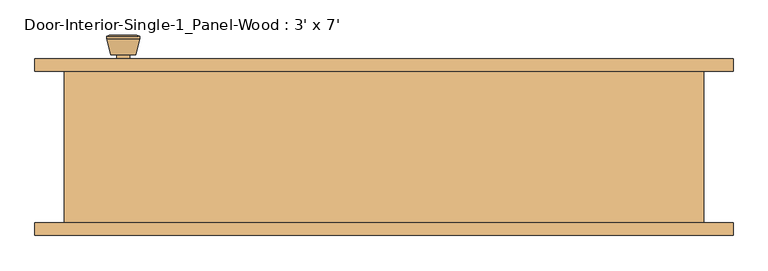
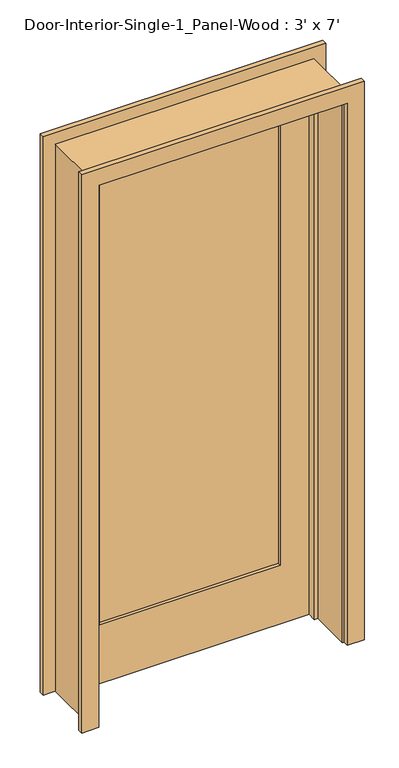
"""IFC4 building model written with IfcOpenShell, lengths in millimetres: door geometry, Door-Interior-Single-1_Panel-Wood : 3' x 7'."""

from ifc_helpers import new_model, si_unit, point, frame, frame_2d, origin, place, context, project, spatial, polyline, circle_curve, trimmed, segment, composite_curve, outline, extrude, faceted_brep, source, transform, mapped, element, save
from ifc_brep_helpers import plane_surface, cylinder_surface, revolved_surface, advanced_brep


def door_interior_single_1_panel_wood_3_x_7_3b97b8e7(model_context):
    return source(origin(), model_context, "Body", "SolidModel", [
        advanced_brep(
        [(-393.7, 70.2, 914.4), (-383.7, 70.2, 914.4), (-403.7, 70.2, 914.4), (-373.2241324, 21.2, 914.4), (-393.7, 21.2, 914.4), (-414.1758676, 21.2, 914.4), (-368.7, 23.0278681, 914.4), (-418.7, 23.0278681, 914.4), (-368.7, 26.4915463, 914.4), (-418.7, 26.4915463, 914.4), (-375.063764, 51.2, 914.4), (-412.336236, 51.2, 914.4), (-383.7, 51.2, 914.4), (-403.7, 51.2, 914.4)],
        [
            (0, 1),
            (1, 2, circle_curve(frame((-393.7, 70.2, 914.4), z_axis=(0.0, 1.0, 0.0), x_axis=(-1.0, 0.0, 0.0)), 10.0)),
            (2, 0),
            (2, 1, circle_curve(frame((-393.7, 70.2, 914.4), z_axis=(0.0, 1.0, 0.0), x_axis=(-1.0, 0.0, 0.0)), 10.0)),
            (3, 4),
            (4, 5),
            (5, 3, circle_curve(frame((-393.7, 21.2, 914.4), z_axis=(0.0, -1.0, 0.0), x_axis=(-1.0, 0.0, 0.0)), 20.4758676)),
            (3, 5, circle_curve(frame((-393.7, 21.2, 914.4), z_axis=(0.0, -1.0, 0.0), x_axis=(-1.0, 0.0, 0.0)), 20.4758676)),
            (6, 3),
            (5, 7),
            (7, 6, circle_curve(frame((-393.7, 23.0278681, 914.4), z_axis=(0.0, -1.0, 0.0), x_axis=(-1.0, 0.0, 0.0)), 25.0)),
            (6, 7, circle_curve(frame((-393.7, 23.0278681, 914.4), z_axis=(0.0, -1.0, 0.0), x_axis=(-1.0, 0.0, 0.0)), 25.0)),
            (8, 6),
            (7, 9),
            (9, 8, circle_curve(frame((-393.7, 26.4915463, 914.4), z_axis=(0.0, -1.0, 0.0), x_axis=(-1.0, 0.0, 0.0)), 25.0)),
            (8, 9, circle_curve(frame((-393.7, 26.4915463, 914.4), z_axis=(0.0, -1.0, 0.0), x_axis=(-1.0, 0.0, 0.0)), 25.0)),
            (10, 8),
            (9, 11),
            (11, 10, circle_curve(frame((-393.7, 51.2, 914.4), z_axis=(0.0, -1.0, 0.0), x_axis=(-1.0, 0.0, 0.0)), 18.636236)),
            (10, 11, circle_curve(frame((-393.7, 51.2, 914.4), z_axis=(0.0, -1.0, 0.0), x_axis=(-1.0, 0.0, 0.0)), 18.636236)),
            (12, 10),
            (11, 13),
            (13, 12, circle_curve(frame((-393.7, 51.2, 914.4), z_axis=(0.0, -1.0, 0.0), x_axis=(-1.0, 0.0, 0.0)), 10.0)),
            (12, 13, circle_curve(frame((-393.7, 51.2, 914.4), z_axis=(0.0, -1.0, 0.0), x_axis=(-1.0, 0.0, 0.0)), 10.0)),
            (1, 12),
            (13, 2),
        ],
        [
            plane_surface(frame((-393.7, 70.2, 914.4), z_axis=(0.0, 1.0, 0.0), x_axis=(-1.0, 0.0, 0.0))),
            plane_surface(frame((-393.7, 21.2, 914.4), z_axis=(0.0, -1.0, 0.0), x_axis=(-1.0, 0.0, 0.0))),
            revolved_surface(polyline([(-414.1758676, 21.2, 914.4), (-418.7, 23.0278681, 914.4)]), (-393.7, 70.2, 914.4), (0.0, 1.0, 0.0)),
            cylinder_surface(frame((-393.7, 70.2, 914.4), z_axis=(0.0, 1.0, 0.0), x_axis=(-1.0, 0.0, 0.0)), 25.0),
            revolved_surface(polyline([(-418.7, 26.4915463, 914.4), (-412.336236, 51.2, 914.4)]), (-393.7, 70.2, 914.4), (0.0, 1.0, 0.0)),
            plane_surface(frame((-393.7, 51.2, 914.4), z_axis=(0.0, 1.0, 0.0), x_axis=(-1.0, 0.0, 0.0))),
            cylinder_surface(frame((-393.7, 70.2, 914.4), z_axis=(0.0, 1.0, 0.0), x_axis=(-1.0, 0.0, 0.0)), 10.0),
        ],
        [
            (0, [[1, 2, 3]]),
            (0, [[-3, 4, -1]]),
            (1, [[5, 6, 7]]),
            (1, [[-6, -5, 8]]),
            (2, [[9, -7, 10, 11]]),
            (2, [[-10, -8, -9, 12]]),
            (3, [[13, -11, 14, 15]]),
            (3, [[-14, -12, -13, 16]]),
            (4, [[17, -15, 18, 19]]),
            (4, [[-18, -16, -17, 20]]),
            (5, [[21, -19, 22, 23]]),
            (5, [[-22, -20, -21, 24]]),
            (6, [[25, -23, 26, -2]]),
            (6, [[-26, -24, -25, -4]]),
        ],
    ),
        extrude(outline(composite_curve([segment(trimmed(circle_curve(frame_2d((914.4, -393.7)), 30.0), [point((914.4, -423.7))], [point((914.4, -363.7))], False, "CARTESIAN"), True, "CONTINUOUS"), segment(trimmed(circle_curve(frame_2d((914.4, -393.7)), 30.0), [point((914.4, -363.7))], [point((914.4, -423.7))], False, "CARTESIAN"), True, "CONTINUOUS")], self_intersect=False)), frame((0.0, 70.2, 0.0), z_axis=(0.0, 1.0, 0.0), x_axis=(0.0, 0.0, 1.0)), (0.0, 0.0, 1.0), 6.0),
        advanced_brep(
        [(-393.7, 117.125, 914.4), (-403.7, 117.125, 914.4), (-383.7, 117.125, 914.4), (-373.2241324, 166.125, 914.4), (-414.1758676, 166.125, 914.4), (-393.7, 166.125, 914.4), (-368.7, 164.2971319, 914.4), (-418.7, 164.2971319, 914.4), (-368.7, 160.8334537, 914.4), (-418.7, 160.8334537, 914.4), (-375.063764, 136.125, 914.4), (-412.336236, 136.125, 914.4), (-383.7, 136.125, 914.4), (-403.7, 136.125, 914.4)],
        [
            (0, 1),
            (1, 2, circle_curve(frame((-393.7, 117.125, 914.4), z_axis=(0.0, -1.0, 0.0), x_axis=(-1.0, 0.0, 0.0)), 10.0)),
            (2, 0),
            (2, 1, circle_curve(frame((-393.7, 117.125, 914.4), z_axis=(0.0, -1.0, 0.0), x_axis=(-1.0, 0.0, 0.0)), 10.0)),
            (3, 4, circle_curve(frame((-393.7, 166.125, 914.4), z_axis=(0.0, 1.0, 0.0), x_axis=(-1.0, 0.0, 0.0)), 20.4758676)),
            (4, 5),
            (5, 3),
            (4, 3, circle_curve(frame((-393.7, 166.125, 914.4), z_axis=(0.0, 1.0, 0.0), x_axis=(-1.0, 0.0, 0.0)), 20.4758676)),
            (6, 7, circle_curve(frame((-393.7, 164.2971319, 914.4), z_axis=(0.0, 1.0, 0.0), x_axis=(-1.0, 0.0, 0.0)), 25.0)),
            (7, 4),
            (3, 6),
            (7, 6, circle_curve(frame((-393.7, 164.2971319, 914.4), z_axis=(0.0, 1.0, 0.0), x_axis=(-1.0, 0.0, 0.0)), 25.0)),
            (8, 9, circle_curve(frame((-393.7, 160.8334537, 914.4), z_axis=(0.0, 1.0, 0.0), x_axis=(-1.0, 0.0, 0.0)), 25.0)),
            (9, 7),
            (6, 8),
            (9, 8, circle_curve(frame((-393.7, 160.8334537, 914.4), z_axis=(0.0, 1.0, 0.0), x_axis=(-1.0, 0.0, 0.0)), 25.0)),
            (10, 11, circle_curve(frame((-393.7, 136.125, 914.4), z_axis=(0.0, 1.0, 0.0), x_axis=(-1.0, 0.0, 0.0)), 18.636236)),
            (11, 9),
            (8, 10),
            (11, 10, circle_curve(frame((-393.7, 136.125, 914.4), z_axis=(0.0, 1.0, 0.0), x_axis=(-1.0, 0.0, 0.0)), 18.636236)),
            (12, 13, circle_curve(frame((-393.7, 136.125, 914.4), z_axis=(0.0, 1.0, 0.0), x_axis=(-1.0, 0.0, 0.0)), 10.0)),
            (13, 11),
            (10, 12),
            (13, 12, circle_curve(frame((-393.7, 136.125, 914.4), z_axis=(0.0, 1.0, 0.0), x_axis=(-1.0, 0.0, 0.0)), 10.0)),
            (1, 13),
            (12, 2),
        ],
        [
            plane_surface(frame((-393.7, 117.125, 914.4), z_axis=(0.0, -1.0, 0.0), x_axis=(-1.0, 0.0, 0.0))),
            plane_surface(frame((-393.7, 166.125, 914.4), z_axis=(0.0, 1.0, 0.0), x_axis=(-1.0, 0.0, 0.0))),
            revolved_surface(polyline([(-414.1758676, 166.125, 914.4), (-418.7, 164.2971319, 914.4)]), (-393.7, 117.125, 914.4), (0.0, -1.0, 0.0)),
            cylinder_surface(frame((-393.7, 117.125, 914.4), z_axis=(0.0, -1.0, 0.0), x_axis=(-1.0, 0.0, 0.0)), 25.0),
            revolved_surface(polyline([(-418.7, 160.8334537, 914.4), (-412.336236, 136.125, 914.4)]), (-393.7, 117.125, 914.4), (0.0, -1.0, 0.0)),
            plane_surface(frame((-393.7, 136.125, 914.4), z_axis=(0.0, -1.0, 0.0), x_axis=(-1.0, 0.0, 0.0))),
            cylinder_surface(frame((-393.7, 117.125, 914.4), z_axis=(0.0, -1.0, 0.0), x_axis=(-1.0, 0.0, 0.0)), 10.0),
        ],
        [
            (0, [[1, 2, 3]]),
            (0, [[-3, 4, -1]]),
            (1, [[5, 6, 7]]),
            (1, [[8, -7, -6]]),
            (2, [[9, 10, -5, 11]]),
            (2, [[12, -11, -8, -10]]),
            (3, [[13, 14, -9, 15]]),
            (3, [[16, -15, -12, -14]]),
            (4, [[17, 18, -13, 19]]),
            (4, [[20, -19, -16, -18]]),
            (5, [[21, 22, -17, 23]]),
            (5, [[24, -23, -20, -22]]),
            (6, [[-2, 25, -21, 26]]),
            (6, [[-4, -26, -24, -25]]),
        ],
    ),
        extrude(outline(composite_curve([segment(trimmed(circle_curve(frame_2d((914.4, -393.7)), 30.0), [point((914.4, -423.7))], [point((914.4, -363.7))], False, "CARTESIAN"), True, "CONTINUOUS"), segment(trimmed(circle_curve(frame_2d((914.4, -393.7)), 30.0), [point((914.4, -363.7))], [point((914.4, -423.7))], False, "CARTESIAN"), True, "CONTINUOUS")], self_intersect=False)), frame((0.0, 111.125, 0.0), z_axis=(0.0, 1.0, 0.0), x_axis=(0.0, 0.0, 1.0)), (0.0, 0.0, 1.0), 6.0),
        faceted_brep([(482.6, 111.125, 0.0), (482.6, -117.475, 0.0), (457.2, -117.475, 0.0), (457.2, 41.275, 0.0), (444.5, 41.275, 0.0), (444.5, 76.2, 0.0), (457.2, 76.2, 0.0), (457.2, 111.125, 0.0), (482.6, 111.125, 2159.0), (482.6, -117.475, 2159.0), (-482.6, -117.475, 2159.0), (-482.6, -117.475, 0.0), (-457.2, -117.475, 0.0), (-457.2, -117.475, 2133.6), (457.2, -117.475, 2133.6), (457.2, 41.275, 2133.6), (-457.2, 41.275, 2133.6), (-457.2, 41.275, 0.0), (-444.5, 41.275, 0.0), (-444.5, 41.275, 2120.9), (444.5, 41.275, 2120.9), (444.5, 76.2, 2120.9), (-444.5, 76.2, 2120.9), (-444.5, 76.2, 0.0), (-457.2, 76.2, 0.0), (-457.2, 76.2, 2133.6), (457.2, 76.2, 2133.6), (457.2, 111.125, 2133.6), (-457.2, 111.125, 2133.6), (-457.2, 111.125, 0.0), (-482.6, 111.125, 0.0), (-482.6, 111.125, 2159.0)], [[[0, 1, 2, 3, 4, 5, 6, 7]], [[1, 0, 8, 9]], [[2, 1, 9, 10, 11, 12, 13, 14]], [[3, 2, 14, 15]], [[4, 3, 15, 16, 17, 18, 19, 20]], [[5, 4, 20, 21]], [[6, 5, 21, 22, 23, 24, 25, 26]], [[7, 6, 26, 27]], [[0, 7, 27, 28, 29, 30, 31, 8]], [[9, 8, 31, 10]], [[15, 14, 13, 16]], [[21, 20, 19, 22]], [[27, 26, 25, 28]], [[30, 29, 24, 23, 18, 17, 12, 11]], [[10, 31, 30, 11]], [[16, 13, 12, 17]], [[22, 19, 18, 23]], [[28, 25, 24, 29]]]),
        extrude(outline(polyline([(2133.6, -457.2), (0.0, -457.2), (0.0, 457.2), (2133.6, 457.2), (2133.6, -457.2)]), holes=[polyline([(2014.5375, -336.55), (2014.5375, 336.55), (231.775, 336.55), (231.775, -336.55), (2014.5375, -336.55)])]), frame((0.0, 76.2, 0.0), z_axis=(0.0, 1.0, 0.0), x_axis=(0.0, 0.0, 1.0)), (0.0, 0.0, 1.0), 34.925),
        extrude(outline(polyline([(336.55, 87.8416667), (-336.55, 87.8416667), (-336.55, 99.4833333), (336.55, 99.4833333), (336.55, 87.8416667)])), frame((0.0, 0.0, 231.775), z_axis=(0.0, 0.0, 1.0), x_axis=(1.0, 0.0, 0.0)), (0.0, 0.0, 1.0), 1782.7625),
        extrude(outline(polyline([(0.0, 463.55), (0.0, 527.05), (2203.45, 527.05), (2203.45, -527.05), (0.0, -527.05), (0.0, -463.55), (2139.95, -463.55), (2139.95, 463.55), (0.0, 463.55)])), frame((0.0, 111.125, 0.0), z_axis=(0.0, 1.0, 0.0), x_axis=(0.0, 0.0, 1.0)), (0.0, 0.0, 1.0), 19.05),
        extrude(outline(polyline([(0.0, 463.55), (0.0, 527.05), (2203.45, 527.05), (2203.45, -527.05), (0.0, -527.05), (0.0, -463.55), (2139.95, -463.55), (2139.95, 463.55), (0.0, 463.55)])), frame((0.0, -136.525, 0.0), z_axis=(0.0, 1.0, 0.0), x_axis=(0.0, 0.0, 1.0)), (0.0, 0.0, 1.0), 19.05),
    ])


if __name__ == "__main__":
    model = new_model("IFC4")
    model_context = context("Model", 3, world=origin())
    ifc_project = project(units=[si_unit("LENGTHUNIT", "METRE", prefix="MILLI")], contexts=[model_context])
    site = spatial("IfcSite", under=ifc_project)
    building = spatial("IfcBuilding", under=site)
    placement = place(None, origin())
    door_interior_single_1_panel_wood_3_x_7_shape = door_interior_single_1_panel_wood_3_x_7_3b97b8e7(model_context)
    element("IfcDoor", 1, ObjectType="Door-Interior-Single-1_Panel-Wood : 3' x 7'", at=placement, inside=building, context=model_context, shape_type="MappedRepresentation", body=[
        mapped(door_interior_single_1_panel_wood_3_x_7_shape, transform((0.0, 0.0, 0.0), x_axis=(1.0, 0.0, 0.0), y_axis=(0.0, 1.0, 0.0), z_axis=(0.0, 0.0, 1.0))),
    ])
    save(model, "model.ifc")

# Revit data of these elements
# Type "Door-Interior-Single-1_Panel-Wood : 3' x 7'"
#   Type Mark = "9"
#   Assembly Code = "C1020300"
#   Analytic Construction = "Wooden"
#   Top Rail = 0' - 4 11/16"
#   Thickness = 0' - 1 3/8"
#   Thermal Resistance (R) = 2.5876 (h·ft²·°F)/BTU
#   Swing Angle [instance default] = 90.00°
#   Stiles = 0' - 4 3/4"
#   Rough Width = 3' - 2"
#   Rough Height = 7' - 1"
#   Height = 7' - 0"
#   Width = 3' - 0"
#   Heat Transfer Coefficient (U) = 0.3865 BTU/(h·ft²·°F)
#   Bottom Rail = 0' - 9 1/8"
#   Trim Material = Cherry
#   Panel Material = Cherry
#   Frame Material = Cherry
#   Door Handle Material = Aluminum
#   Visual Light Transmittance = 0
#   Solar Heat Gain Coefficient = 0
#   Wall Closure = (empty or 0)
#   Function = (empty or 0)
# Element 1 (IfcDoor, "Door-Interior-Single-1_Panel-Wood : 3' x 7'")
#   Materials on its faces: "Cherry", "Aluminum"
# Materials
#   "Cherry": class "Wood", colour RGB 226 177 128, transparency 0, Description = "Prunus Serotina", Cost = 0
#   "Aluminum": class "Metal", colour RGB 247 247 247, transparency 0, Description = "Aluminum 6061", Cost = 0
